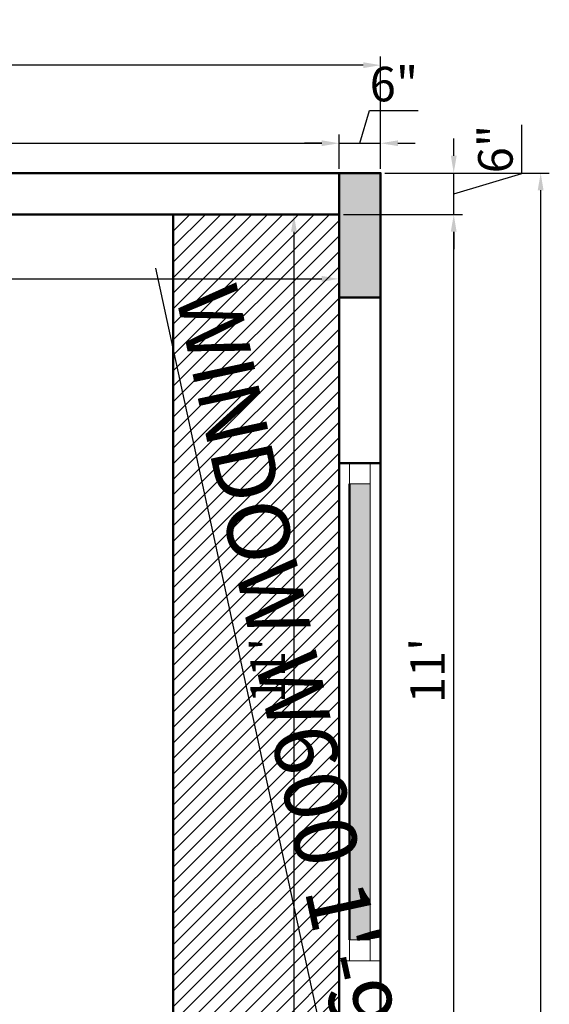
# Model space of a CAD drawing. Units: inches. Extents: x 3064 to 19385, y 846 to 15425.
# Tile 107 of 108: x 7816 to 7893, y 1276 to 1419. Entities that reach past the tile are written whole.
import ezdxf

# ---------------------------------------------------------------- set-up
doc = ezdxf.new("R2010")
doc.units = ezdxf.units.IN
for name, color, linetype, lineweight in [('A-ANNO-DIMS', 2, 'Continuous', 18), ('A-COLS', 1, 'Continuous', 35), ('A-FURN-PATT', 252, 'Continuous', 13), ('A-GLAZ', 4, 'Continuous', 18), ('A-WALL', 7, 'Continuous', 50)]:
    doc.layers.add(name, color=color, linetype=linetype, lineweight=lineweight)
doc.styles.get("Standard").update_dxf_attribs({"font": 'arial.ttf'})
doc.dimstyles.new('ISO-25', dxfattribs={"dimtxt": 9, "dimasz": 2.5, "dimexe": 1.25, "dimexo": 0.625, "dimtad": 1, "dimdec": 1, "dimlunit": 3, "dimtxsty": 'Standard', "dimcen": 2.5, "dimadec": 0, "dimazin": 0, "dimtfac": 1, "dimtdec": 1, "dimtmove": 0, "dimatfit": 3, "dimfxl": 1, "dimarcsym": 0})

# ---------------------------------------------------------------- blocks, each defined once
blk = doc.blocks.new('*D333')
at = {"layer": 'A-ANNO-DIMS', "color": 0, "lineweight": -2, "transparency": 16777216}
for p, q in [((7862.87, 1390.34), (7880.08, 1390.34)), ((7878.83, 1260.84), (7878.83, 1387.84)), ((7868.87, 1258.34), (7880.08, 1258.34))]:
    blk.add_line(p, q, dxfattribs=at)
at = {"layer": 'A-ANNO-DIMS', "color": 0, "transparency": 16777216}
for points in [[(7878.41, 1387.84), (7879.25, 1387.84), (7878.83, 1390.34)], [(7878.41, 1260.84), (7879.25, 1260.84), (7878.83, 1258.34)]]:
    blk.add_solid(points, dxfattribs=at)
at = {"layer": 'Defpoints', "color": 0, "transparency": 16777216}
for p in [(7862.25, 1390.34), (7878.83, 1390.34), (7868.25, 1258.34)]:
    blk.add_point(p, dxfattribs=at)
at = {"layer": 'A-ANNO-DIMS', "color": 0, "transparency": 16777216, "insert": (7875.69, 1324.34), "char_height": 5, "attachment_point": 5, "rotation": 90}
blk.add_mtext("11'", dxfattribs=at)
blk = doc.blocks.new('*D334')
at = {"layer": 'A-ANNO-DIMS', "color": 0, "lineweight": -2, "transparency": 16777216}
for p, q in [((7888.67, 1396.29), (7888.67, 1403.32)), ((7878.83, 1398.84), (7878.83, 1401.34)), ((7868.87, 1396.34), (7880.08, 1396.34)), ((7878.83, 1390.34), (7878.83, 1396.34)), ((7878.83, 1390.34), (7878.83, 1396.34)), ((7878.83, 1393.34), (7888.67, 1396.29)), ((7862.87, 1390.34), (7880.08, 1390.34)), ((7878.83, 1387.84), (7878.83, 1385.34))]:
    blk.add_line(p, q, dxfattribs=at)
at = {"layer": 'A-ANNO-DIMS', "color": 0, "transparency": 16777216}
for points in [[(7878.41, 1398.84), (7879.25, 1398.84), (7878.83, 1396.34)], [(7878.41, 1387.84), (7879.25, 1387.84), (7878.83, 1390.34)]]:
    blk.add_solid(points, dxfattribs=at)
at = {"layer": 'Defpoints', "color": 0, "transparency": 16777216}
for p in [(7868.25, 1396.34), (7878.83, 1396.34), (7862.25, 1390.34)]:
    blk.add_point(p, dxfattribs=at)
at = {"layer": 'A-ANNO-DIMS', "color": 0, "transparency": 16777216, "insert": (7885.5, 1399.81), "char_height": 5, "attachment_point": 5, "rotation": 90}
blk.add_mtext('6"', dxfattribs=at)
blk = doc.blocks.new('*D335')
at = {"layer": 'A-ANNO-DIMS', "color": 0, "lineweight": -2, "transparency": 16777216}
for p, q in [((7868.87, 1396.34), (7892.65, 1396.34)), ((7891.4, 1393.84), (7891.4, 906.84)), ((7868.87, 904.34), (7892.65, 904.34))]:
    blk.add_line(p, q, dxfattribs=at)
at = {"layer": 'A-ANNO-DIMS', "color": 0, "transparency": 16777216}
for points in [[(7890.98, 1393.84), (7891.82, 1393.84), (7891.4, 1396.34)], [(7890.98, 906.84), (7891.82, 906.84), (7891.4, 904.34)]]:
    blk.add_solid(points, dxfattribs=at)
at = {"layer": 'Defpoints', "color": 0, "transparency": 16777216}
for p in [(7868.25, 1396.34), (7868.25, 904.34), (7891.4, 904.34)]:
    blk.add_point(p, dxfattribs=at)
at = {"layer": 'A-ANNO-DIMS', "color": 0, "transparency": 16777216, "insert": (7888.27, 1150.34), "char_height": 5, "attachment_point": 5, "rotation": 90}
blk.add_mtext("41'", dxfattribs=at)
blk = doc.blocks.new('*D338')
at = {"layer": 'A-ANNO-DIMS', "color": 0, "lineweight": -2, "transparency": 16777216}
for p, q in [((7667.25, 1396.96), (7667.25, 1401.9)), ((7862.25, 1396.96), (7862.25, 1401.9)), ((7669.75, 1400.65), (7859.75, 1400.65))]:
    blk.add_line(p, q, dxfattribs=at)
at = {"layer": 'A-ANNO-DIMS', "color": 0, "transparency": 16777216}
for points in [[(7669.75, 1401.07), (7669.75, 1400.24), (7667.25, 1400.65)], [(7859.75, 1401.07), (7859.75, 1400.24), (7862.25, 1400.65)]]:
    blk.add_solid(points, dxfattribs=at)
at = {"layer": 'Defpoints', "color": 0, "transparency": 16777216}
for p in [(7862.25, 1400.65), (7667.25, 1396.34), (7862.25, 1396.34)]:
    blk.add_point(p, dxfattribs=at)
at = {"layer": 'A-ANNO-DIMS', "color": 0, "transparency": 16777216, "insert": (7764.75, 1403.83), "char_height": 5, "attachment_point": 5}
blk.add_mtext('16\'-3"', dxfattribs=at)
blk = doc.blocks.new('*D339')
at = {"layer": 'A-ANNO-DIMS', "color": 0, "lineweight": -2, "transparency": 16777216}
for p, q in [((7865.25, 1400.65), (7866.67, 1405.39)), ((7866.67, 1405.39), (7873.69, 1405.39)), ((7862.25, 1396.96), (7862.25, 1401.9)), ((7868.25, 1396.96), (7868.25, 1401.9)), ((7859.75, 1400.65), (7857.25, 1400.65)), ((7862.25, 1400.65), (7868.25, 1400.65)), ((7862.25, 1400.65), (7868.25, 1400.65)), ((7870.75, 1400.65), (7873.25, 1400.65))]:
    blk.add_line(p, q, dxfattribs=at)
at = {"layer": 'A-ANNO-DIMS', "color": 0, "transparency": 16777216}
for points in [[(7859.75, 1401.07), (7859.75, 1400.24), (7862.25, 1400.65)], [(7870.75, 1401.07), (7870.75, 1400.24), (7868.25, 1400.65)]]:
    blk.add_solid(points, dxfattribs=at)
at = {"layer": 'Defpoints', "color": 0, "transparency": 16777216}
for p in [(7868.25, 1400.65), (7862.25, 1396.34), (7868.25, 1396.34)]:
    blk.add_point(p, dxfattribs=at)
at = {"layer": 'A-ANNO-DIMS', "color": 0, "transparency": 16777216, "insert": (7870.18, 1408.57), "char_height": 5, "attachment_point": 5}
blk.add_mtext('6"', dxfattribs=at)
blk = doc.blocks.new('*D226')
at = {"layer": 'A-ANNO-DIMS', "color": 0, "lineweight": -2, "transparency": 16777216}
for p, q in [((7526.25, 1396.96), (7526.25, 1413.2)), ((7868.25, 1396.96), (7868.25, 1413.2)), ((7865.75, 1411.95), (7528.75, 1411.95))]:
    blk.add_line(p, q, dxfattribs=at)
at = {"layer": 'A-ANNO-DIMS', "color": 0, "transparency": 16777216}
for points in [[(7528.75, 1412.37), (7528.75, 1411.53), (7526.25, 1411.95)], [(7865.75, 1412.37), (7865.75, 1411.53), (7868.25, 1411.95)]]:
    blk.add_solid(points, dxfattribs=at)
at = {"layer": 'Defpoints', "color": 0, "transparency": 16777216}
for p in [(7526.25, 1411.95), (7526.25, 1396.34), (7868.25, 1396.34)]:
    blk.add_point(p, dxfattribs=at)
at = {"layer": 'A-ANNO-DIMS', "color": 0, "transparency": 16777216, "insert": (7697.25, 1415.13), "char_height": 5, "attachment_point": 5}
blk.add_mtext('28\'-6"', dxfattribs=at)
blk = doc.blocks.new('*D248')
at = {"layer": 'A-ANNO-DIMS', "color": 0, "lineweight": -2, "transparency": 16777216}
for p, q in [((7667.25, 1389.71), (7667.25, 1379.77)), ((7862.25, 1389.71), (7862.25, 1379.77)), ((7669.75, 1381.02), (7859.75, 1381.02))]:
    blk.add_line(p, q, dxfattribs=at)
at = {"layer": 'A-ANNO-DIMS', "color": 0, "transparency": 16777216}
for points in [[(7669.75, 1381.44), (7669.75, 1380.6), (7667.25, 1381.02)], [(7859.75, 1381.44), (7859.75, 1380.6), (7862.25, 1381.02)]]:
    blk.add_solid(points, dxfattribs=at)
at = {"layer": 'Defpoints', "color": 0, "transparency": 16777216}
for p in [(7667.25, 1390.34), (7862.25, 1390.34), (7862.25, 1381.02)]:
    blk.add_point(p, dxfattribs=at)
at = {"layer": 'A-ANNO-DIMS', "color": 0, "transparency": 16777216, "insert": (7764.75, 1384.2), "char_height": 5, "attachment_point": 5}
blk.add_mtext('16\'-3"', dxfattribs=at)
blk = doc.blocks.new('*D249')
at = {"layer": 'A-ANNO-DIMS', "color": 0, "lineweight": -2, "transparency": 16777216}
for p, q in [((7861.62, 1390.34), (7854.47, 1390.34)), ((7855.72, 1387.84), (7855.72, 1260.84)), ((7861.62, 1258.34), (7854.47, 1258.34))]:
    blk.add_line(p, q, dxfattribs=at)
at = {"layer": 'A-ANNO-DIMS', "color": 0, "transparency": 16777216}
for points in [[(7855.3, 1387.84), (7856.13, 1387.84), (7855.72, 1390.34)], [(7855.3, 1260.84), (7856.13, 1260.84), (7855.72, 1258.34)]]:
    blk.add_solid(points, dxfattribs=at)
at = {"layer": 'Defpoints', "color": 0, "transparency": 16777216}
for p in [(7862.25, 1390.34), (7855.72, 1258.34), (7862.25, 1258.34)]:
    blk.add_point(p, dxfattribs=at)
at = {"layer": 'A-ANNO-DIMS', "color": 0, "transparency": 16777216, "insert": (7852.58, 1324.34), "char_height": 5, "attachment_point": 5, "rotation": 90}
blk.add_mtext("11'", dxfattribs=at)
blk = doc.blocks.new('WIN-1900')
blk.add_line((3, 0), (3, 66))
blk.add_lwpolyline([(3, 66), (0, 66), (0, 69), (3, 69)], close=True)
blk = doc.blocks.new('*D439')
at = {"layer": 'A-ANNO-DIMS', "color": 0, "lineweight": -2, "transparency": 16777216}
for p, q in [((7868.32, 1232.06), (7835.74, 1382.55)), ((7865.85, 1231.53), (7869.54, 1232.32)), ((7872.24, 1213.98), (7868.85, 1229.62)), ((7870.3, 1211), (7873.99, 1211.8))]:
    blk.add_line(p, q, dxfattribs=at)
at = {"layer": 'A-ANNO-DIMS', "color": 0, "transparency": 16777216}
for points in [[(7869.26, 1229.7), (7868.44, 1229.53), (7868.32, 1232.06)], [(7872.64, 1214.07), (7871.83, 1213.89), (7872.76, 1211.54)]]:
    blk.add_solid(points, dxfattribs=at)
at = {"layer": 'Defpoints', "color": 0, "transparency": 16777216}
for p in [(7865.24, 1231.39), (7868.32, 1232.06), (7869.69, 1210.87)]:
    blk.add_point(p, dxfattribs=at)
at = {"layer": 'A-ANNO-DIMS', "color": 0, "transparency": 16777216, "insert": (7856.93, 1309.64), "char_height": 9, "attachment_point": 5, "rotation": 282.2157}
blk.add_mtext('WINDOW W600 1\'-9" TYP.', dxfattribs=at)

msp = doc.modelspace()

# ---------------------------------------------------------------- hatches: boundary and pattern name
at = {"layer": 'A-COLS'}
h = msp.add_hatch(color=256, dxfattribs=at)
h.dxf.hatch_style = 1
h.paths.add_polyline_path([(7862.25, 1378.34), (7868.25, 1378.34), (7868.25, 1396.34), (7862.25, 1396.34)])
at = {"layer": 'A-FURN-PATT'}
h = msp.add_hatch(dxfattribs=at)
h.set_pattern_fill('ANSI31', color=256, scale=0.5)
h.set_pattern_definition([(45, (3183.7531, 0), (-1.122532, 1.122532), [])])
h.paths.add_polyline_path([(7838.25, 1258.34), (7862.25, 1258.34), (7862.25, 1390.34), (7838.25, 1390.34)])
at = {"layer": 'A-GLAZ'}
h = msp.add_hatch(color=256, dxfattribs=at)
h.dxf.hatch_style = 1
h.paths.add_polyline_path([(7863.75, 1285.34), (7866.75, 1285.34), (7866.75, 1351.34), (7863.75, 1351.34)])

# ---------------------------------------------------------------- linework, layer by layer
msp.add_line((7868.25, 1282.34), (7862.25, 1282.34), dxfattribs=at)
msp.add_lwpolyline([(7866.75, 1282.34), (7863.75, 1282.34), (7863.75, 1285.34), (7866.75, 1285.34)], close=True, dxfattribs=at)
at = {"layer": 'A-WALL'}
for p, q in [((7868.25, 1396.34), (7526.25, 1396.34)), ((7868.25, 904.34), (7868.25, 1396.34)), ((7862.25, 1390.34), (7667.25, 1390.34)), ((7838.25, 1258.34), (7838.25, 1390.34)), ((7862.25, 1258.34), (7862.25, 1390.34)), ((7862.25, 1354.34), (7868.25, 1354.34)), ((7863.75, 1351.34), (7863.75, 1285.34))]:
    msp.add_line(p, q, dxfattribs=at)
msp.add_lwpolyline([(7868.25, 1378.34), (7868.25, 1396.34), (7862.25, 1396.34), (7862.25, 1378.34)], close=True, dxfattribs=at)

# ---------------------------------------------------------------- block references
at = {"layer": 'A-GLAZ'}
msp.add_blockref('WIN-1900', (7863.75, 1285.34), dxfattribs=at)

# ---------------------------------------------------------------- dimensions: what is measured, and where the dimension line sits
at = {"layer": 'A-ANNO-DIMS'}
for base, p1, p2, override, picture, middle in [((7526.25, 1411.95), (7868.25, 1396.34), (7526.25, 1396.34), {"dimtxt": 5, "dimclrd": 0, "dimclre": 0, "dimclrt": 0}, '*D226', (7697.25, 1415.13)), ((7868.25, 1400.65), (7862.25, 1396.34), (7868.25, 1396.34), {"dimtxt": 5, "dimclrd": 0, "dimclre": 0, "dimclrt": 0, "dimtmove": 1}, '*D339', (7867.29, 1408.57)), ((7862.25, 1400.65), (7667.25, 1396.34), (7862.25, 1396.34), {"dimtxt": 5, "dimclrd": 0, "dimclre": 0, "dimclrt": 0, "dimtmove": 1}, '*D338', (7764.75, 1403.83)), ((7862.25, 1381.02), (7667.25, 1390.34), (7862.25, 1390.34), {"dimtxt": 5, "dimclrd": 0, "dimclre": 0, "dimclrt": 0}, '*D248', (7764.75, 1384.2))]:
    dim = msp.add_linear_dim(base=base, p1=p1, p2=p2, dimstyle='ISO-25', override=override, dxfattribs=at)
    dim.commit()
    dim.dimension.update_dxf_attribs({"geometry": picture, "text_midpoint": middle})
for base, p1, p2, override, picture, middle in [((7878.83, 1396.34), (7862.25, 1390.34), (7868.25, 1396.34), {"dimtxt": 5, "dimclrd": 0, "dimclre": 0, "dimclrt": 0, "dimtmove": 1}, '*D334', (7885.5, 1396.92)), ((7891.4, 904.34), (7868.25, 1396.34), (7868.25, 904.34), {"dimtxt": 5, "dimclrd": 0, "dimclre": 0, "dimclrt": 0}, '*D335', (7888.27, 1150.34)), ((7855.72, 1258.34), (7862.25, 1390.34), (7862.25, 1258.34), {"dimtxt": 5, "dimclrd": 0, "dimclre": 0, "dimclrt": 0}, '*D249', (7852.58, 1324.34)), ((7878.83, 1390.34), (7868.25, 1258.34), (7862.25, 1390.34), {"dimtxt": 5, "dimclrd": 0, "dimclre": 0, "dimclrt": 0, "dimtmove": 1}, '*D333', (7875.69, 1324.34))]:
    dim = msp.add_linear_dim(base=base, p1=p1, p2=p2, angle=90, dimstyle='ISO-25', override=override, dxfattribs=at)
    dim.commit()
    dim.dimension.update_dxf_attribs({"geometry": picture, "text_midpoint": middle})
dim = msp.add_linear_dim(base=(7868.32, 1232.06), p1=(7869.69, 1210.87), p2=(7865.24, 1231.39), angle=102.2157, text='WINDOW W600 <> TYP.', dimstyle='ISO-25', override={"dimdec": 1, "dimrnd": 0, "dimzin": 1, "dimlunit": 4, "dimfrac": 2}, dxfattribs=at)
dim.commit()
dim.dimension.update_dxf_attribs({"geometry": '*D439', "text_midpoint": (7856.93, 1309.64)})

doc.saveas('drawing.dxf')
